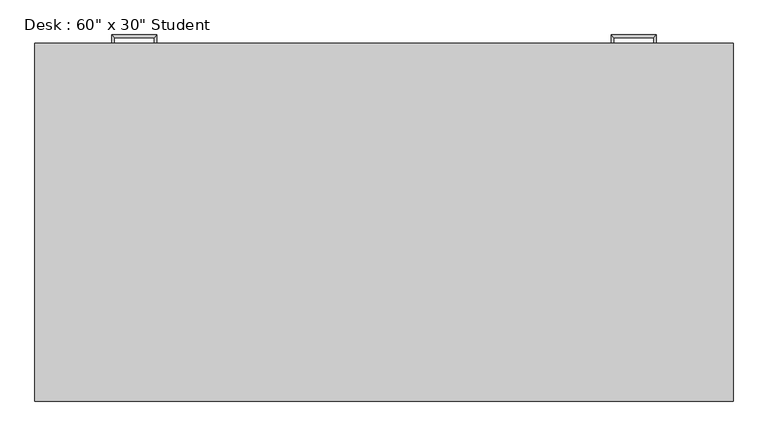
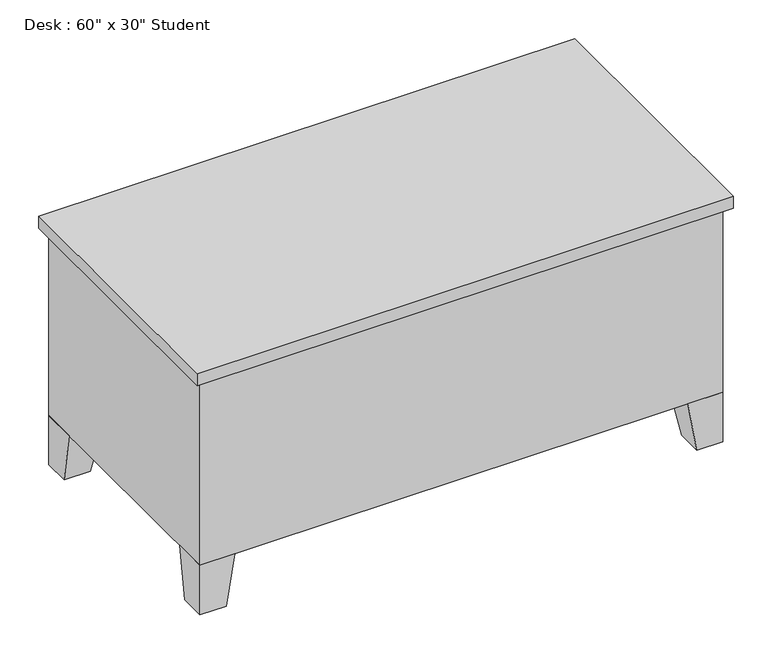
"""IFC4 building model written with IfcOpenShell, lengths in millimetres: furniture geometry."""

from ifc_helpers import new_model, si_unit, frame, origin, place, context, project, spatial, polyline, outline, extrude, faceted_brep, source, transform, mapped, element, save


def furniture_072f6425(model_context):
    return source(origin(), model_context, "Body", "SolidModel", [
        extrude(outline(polyline([(1504.95, 762.0), (1136.65, 762.0), (1136.65, 774.7), (1504.95, 774.7), (1504.95, 762.0)])), frame((0.0, 0.0, 603.25), z_axis=(0.0, 0.0, 1.0), x_axis=(1.0, 0.0, 0.0)), (0.0, 0.0, 1.0), 101.6),
        extrude(outline(polyline([(1504.95, 762.0), (1136.65, 762.0), (1136.65, 774.7), (1504.95, 774.7), (1504.95, 762.0)])), frame((0.0, 0.0, 171.45), z_axis=(0.0, 0.0, 1.0), x_axis=(1.0, 0.0, 0.0)), (0.0, 0.0, 1.0), 412.75),
        extrude(outline(polyline([(387.35, 762.0), (19.05, 762.0), (19.05, 774.7), (387.35, 774.7), (387.35, 762.0)])), frame((0.0, 0.0, 603.25), z_axis=(0.0, 0.0, 1.0), x_axis=(1.0, 0.0, 0.0)), (0.0, 0.0, 1.0), 101.6),
        extrude(outline(polyline([(387.35, 762.0), (19.05, 762.0), (19.05, 774.7), (387.35, 774.7), (387.35, 762.0)])), frame((0.0, 0.0, 171.45), z_axis=(0.0, 0.0, 1.0), x_axis=(1.0, 0.0, 0.0)), (0.0, 0.0, 1.0), 171.45),
        extrude(outline(polyline([(387.35, 762.0), (19.05, 762.0), (19.05, 774.7), (387.35, 774.7), (387.35, 762.0)])), frame((0.0, 0.0, 482.6), z_axis=(0.0, 0.0, 1.0), x_axis=(1.0, 0.0, 0.0)), (0.0, 0.0, 1.0), 101.6),
        extrude(outline(polyline([(387.35, 762.0), (19.05, 762.0), (19.05, 774.7), (387.35, 774.7), (387.35, 762.0)])), frame((0.0, 0.0, 361.95), z_axis=(0.0, 0.0, 1.0), x_axis=(1.0, 0.0, 0.0)), (0.0, 0.0, 1.0), 101.6),
        faceted_brep([(1422.4, 762.0, 152.4), (1422.4, 660.4, 152.4), (1524.0, 660.4, 152.4), (1524.0, 762.0, 152.4), (1447.8, 762.0, 0.0), (1524.0, 762.0, 0.0), (1524.0, 685.8, 0.0), (1447.8, 685.8, 0.0)], [[[0, 1, 2, 3]], [[4, 5, 6, 7]], [[4, 7, 1, 0]], [[7, 6, 2, 1]], [[6, 5, 3, 2]], [[5, 4, 0, 3]]]),
        faceted_brep([(1422.4, 0.0, 152.4), (1524.0, 0.0, 152.4), (1524.0, 101.6, 152.4), (1422.4, 101.6, 152.4), (1447.8, 0.0, 0.0), (1447.8, 76.2, 0.0), (1524.0, 76.2, 0.0), (1524.0, 0.0, 0.0)], [[[0, 1, 2, 3]], [[4, 5, 6, 7]], [[4, 7, 1, 0]], [[7, 6, 2, 1]], [[6, 5, 3, 2]], [[5, 4, 0, 3]]]),
        faceted_brep([(101.6, 0.0, 152.4), (101.6, 101.6, 152.4), (0.0, 101.6, 152.4), (0.0, 0.0, 152.4), (76.2, 0.0, 0.0), (0.0, 0.0, 0.0), (0.0, 76.2, 0.0), (76.2, 76.2, 0.0)], [[[0, 1, 2, 3]], [[4, 5, 6, 7]], [[4, 7, 1, 0]], [[7, 6, 2, 1]], [[6, 5, 3, 2]], [[5, 4, 0, 3]]]),
        faceted_brep([(101.6, 762.0, 152.4), (0.0, 762.0, 152.4), (0.0, 660.4, 152.4), (101.6, 660.4, 152.4), (76.2, 762.0, 0.0), (76.2, 685.8, 0.0), (0.0, 685.8, 0.0), (0.0, 762.0, 0.0)], [[[0, 1, 2, 3]], [[4, 5, 6, 7]], [[4, 7, 1, 0]], [[7, 6, 2, 1]], [[6, 5, 3, 2]], [[5, 4, 0, 3]]]),
        extrude(outline(polyline([(1543.05, 781.05), (1543.05, -19.05), (-19.05, -19.05), (-19.05, 781.05), (1543.05, 781.05)])), frame((0.0, 0.0, 723.9), z_axis=(0.0, 0.0, 1.0), x_axis=(1.0, 0.0, 0.0)), (0.0, 0.0, 1.0), 38.1),
        extrude(outline(polyline([(406.4, 762.0), (406.4, 50.8), (1117.6, 50.8), (1117.6, 762.0), (1524.0, 762.0), (1524.0, 0.0), (0.0, 0.0), (0.0, 762.0), (406.4, 762.0)])), frame((0.0, 0.0, 152.4), z_axis=(0.0, 0.0, 1.0), x_axis=(1.0, 0.0, 0.0)), (0.0, 0.0, 1.0), 571.5),
        faceted_brep([(1365.25, 774.7, 546.1), (1365.25, 774.7, 533.4), (1371.6, 774.7, 533.4), (1371.6, 774.7, 546.1), (1365.25, 793.75, 546.1), (1365.25, 793.75, 533.4), (1371.6, 800.1, 533.4), (1371.6, 800.1, 546.1), (1276.35, 793.75, 546.1), (1276.35, 793.75, 533.4), (1270.0, 800.1, 533.4), (1270.0, 800.1, 546.1), (1276.35, 774.7, 546.1), (1270.0, 774.7, 546.1), (1270.0, 774.7, 533.4), (1276.35, 774.7, 533.4)], [[[0, 1, 2, 3]], [[1, 0, 4, 5]], [[2, 1, 5, 6]], [[3, 2, 6, 7]], [[0, 3, 7, 4]], [[5, 4, 8, 9]], [[6, 5, 9, 10]], [[7, 6, 10, 11]], [[4, 7, 11, 8]], [[12, 13, 14, 15]], [[9, 8, 12, 15]], [[10, 9, 15, 14]], [[11, 10, 14, 13]], [[8, 11, 13, 12]]]),
        faceted_brep([(1365.25, 774.7, 666.75), (1365.25, 774.7, 654.05), (1371.6, 774.7, 654.05), (1371.6, 774.7, 666.75), (1365.25, 793.75, 666.75), (1365.25, 793.75, 654.05), (1371.6, 800.1, 654.05), (1371.6, 800.1, 666.75), (1276.35, 793.75, 666.75), (1276.35, 793.75, 654.05), (1270.0, 800.1, 654.05), (1270.0, 800.1, 666.75), (1276.35, 774.7, 666.75), (1270.0, 774.7, 666.75), (1270.0, 774.7, 654.05), (1276.35, 774.7, 654.05)], [[[0, 1, 2, 3]], [[1, 0, 4, 5]], [[2, 1, 5, 6]], [[3, 2, 6, 7]], [[0, 3, 7, 4]], [[5, 4, 8, 9]], [[6, 5, 9, 10]], [[7, 6, 10, 11]], [[4, 7, 11, 8]], [[12, 13, 14, 15]], [[9, 8, 12, 15]], [[10, 9, 15, 14]], [[11, 10, 14, 13]], [[8, 11, 13, 12]]]),
        faceted_brep([(158.75, 774.7, 304.8), (152.4, 774.7, 304.8), (152.4, 774.7, 292.1), (158.75, 774.7, 292.1), (158.75, 793.75, 304.8), (152.4, 800.1, 304.8), (152.4, 800.1, 292.1), (158.75, 793.75, 292.1), (247.65, 793.75, 304.8), (254.0, 800.1, 304.8), (254.0, 800.1, 292.1), (247.65, 793.75, 292.1), (247.65, 774.7, 304.8), (247.65, 774.7, 292.1), (254.0, 774.7, 292.1), (254.0, 774.7, 304.8)], [[[0, 1, 2, 3]], [[1, 0, 4, 5]], [[2, 1, 5, 6]], [[3, 2, 6, 7]], [[0, 3, 7, 4]], [[5, 4, 8, 9]], [[6, 5, 9, 10]], [[7, 6, 10, 11]], [[4, 7, 11, 8]], [[12, 13, 14, 15]], [[9, 8, 12, 15]], [[10, 9, 15, 14]], [[11, 10, 14, 13]], [[8, 11, 13, 12]]]),
        faceted_brep([(158.75, 774.7, 425.45), (152.4, 774.7, 425.45), (152.4, 774.7, 412.75), (158.75, 774.7, 412.75), (158.75, 793.75, 425.45), (152.4, 800.1, 425.45), (152.4, 800.1, 412.75), (158.75, 793.75, 412.75), (247.65, 793.75, 425.45), (254.0, 800.1, 425.45), (254.0, 800.1, 412.75), (247.65, 793.75, 412.75), (247.65, 774.7, 425.45), (247.65, 774.7, 412.75), (254.0, 774.7, 412.75), (254.0, 774.7, 425.45)], [[[0, 1, 2, 3]], [[1, 0, 4, 5]], [[2, 1, 5, 6]], [[3, 2, 6, 7]], [[0, 3, 7, 4]], [[5, 4, 8, 9]], [[6, 5, 9, 10]], [[7, 6, 10, 11]], [[4, 7, 11, 8]], [[12, 13, 14, 15]], [[9, 8, 12, 15]], [[10, 9, 15, 14]], [[11, 10, 14, 13]], [[8, 11, 13, 12]]]),
        faceted_brep([(158.75, 774.7, 546.1), (152.4, 774.7, 546.1), (152.4, 774.7, 533.4), (158.75, 774.7, 533.4), (158.75, 793.75, 546.1), (152.4, 800.1, 546.1), (152.4, 800.1, 533.4), (158.75, 793.75, 533.4), (247.65, 793.75, 546.1), (254.0, 800.1, 546.1), (254.0, 800.1, 533.4), (247.65, 793.75, 533.4), (247.65, 774.7, 546.1), (247.65, 774.7, 533.4), (254.0, 774.7, 533.4), (254.0, 774.7, 546.1)], [[[0, 1, 2, 3]], [[1, 0, 4, 5]], [[2, 1, 5, 6]], [[3, 2, 6, 7]], [[0, 3, 7, 4]], [[5, 4, 8, 9]], [[6, 5, 9, 10]], [[7, 6, 10, 11]], [[4, 7, 11, 8]], [[12, 13, 14, 15]], [[9, 8, 12, 15]], [[10, 9, 15, 14]], [[11, 10, 14, 13]], [[8, 11, 13, 12]]]),
        faceted_brep([(158.75, 774.7, 666.75), (152.4, 774.7, 666.75), (152.4, 774.7, 654.05), (158.75, 774.7, 654.05), (158.75, 793.75, 666.75), (152.4, 800.1, 666.75), (152.4, 800.1, 654.05), (158.75, 793.75, 654.05), (247.65, 793.75, 666.75), (254.0, 800.1, 666.75), (254.0, 800.1, 654.05), (247.65, 793.75, 654.05), (247.65, 774.7, 666.75), (247.65, 774.7, 654.05), (254.0, 774.7, 654.05), (254.0, 774.7, 666.75)], [[[0, 1, 2, 3]], [[1, 0, 4, 5]], [[2, 1, 5, 6]], [[3, 2, 6, 7]], [[0, 3, 7, 4]], [[5, 4, 8, 9]], [[6, 5, 9, 10]], [[7, 6, 10, 11]], [[4, 7, 11, 8]], [[12, 13, 14, 15]], [[9, 8, 12, 15]], [[10, 9, 15, 14]], [[11, 10, 14, 13]], [[8, 11, 13, 12]]]),
    ])


if __name__ == "__main__":
    model = new_model("IFC4")
    model_context = context("Model", 3, world=origin())
    ifc_project = project(units=[si_unit("LENGTHUNIT", "METRE", prefix="MILLI")], contexts=[model_context])
    site = spatial("IfcSite", under=ifc_project)
    building = spatial("IfcBuilding", under=site)
    placement = place(None, origin())
    furniture_shape = furniture_072f6425(model_context)
    element("IfcFurniture", 1, ObjectType="Desk : 60\" x 30\" Student", at=placement, inside=building, context=model_context, shape_type="MappedRepresentation", body=[
        mapped(furniture_shape, transform((0.0, 0.0, 0.0), x_axis=(1.0, 0.0, 0.0), y_axis=(0.0, 1.0, 0.0), z_axis=(0.0, 0.0, 1.0))),
    ])
    save(model, "model.ifc")

# Revit data of these elements
# Type "Desk : 60\" x 30\" Student"
#   Assembly Code = "E2020200"
#   Depth = 2' - 6"
#   Height = 2' - 6"
#   Leg Height = 0' - 6"
#   Width = 5' - 0"
#   Body Material = Laminate, Ivory, Matte
#   Handle/Leg Material = Steel, Chrome Plated
#   Top Material = Cherry
#   Default Elevation = 0
# Element 1 (IfcFurniture, "Desk : 60\" x 30\" Student")
#   Materials on its faces: "Steel, Chrome Plated", "Laminate, Ivory, Matte", "Cherry"
# Materials
#   "Laminate, Ivory, Matte": class "Plastic", colour RGB 247 247 239, transparency 0, Description = "Plastic Laminate - Ivory, Matte", Cost = 0
#   "Steel, Chrome Plated": class "Metal", colour RGB 17 17 17, transparency 0, Description = "Chromiuim plated steel", Cost = 0
#   "Cherry": class "Wood", colour RGB 226 177 128, transparency 0, Description = "Prunus Serotina", Cost = 0
